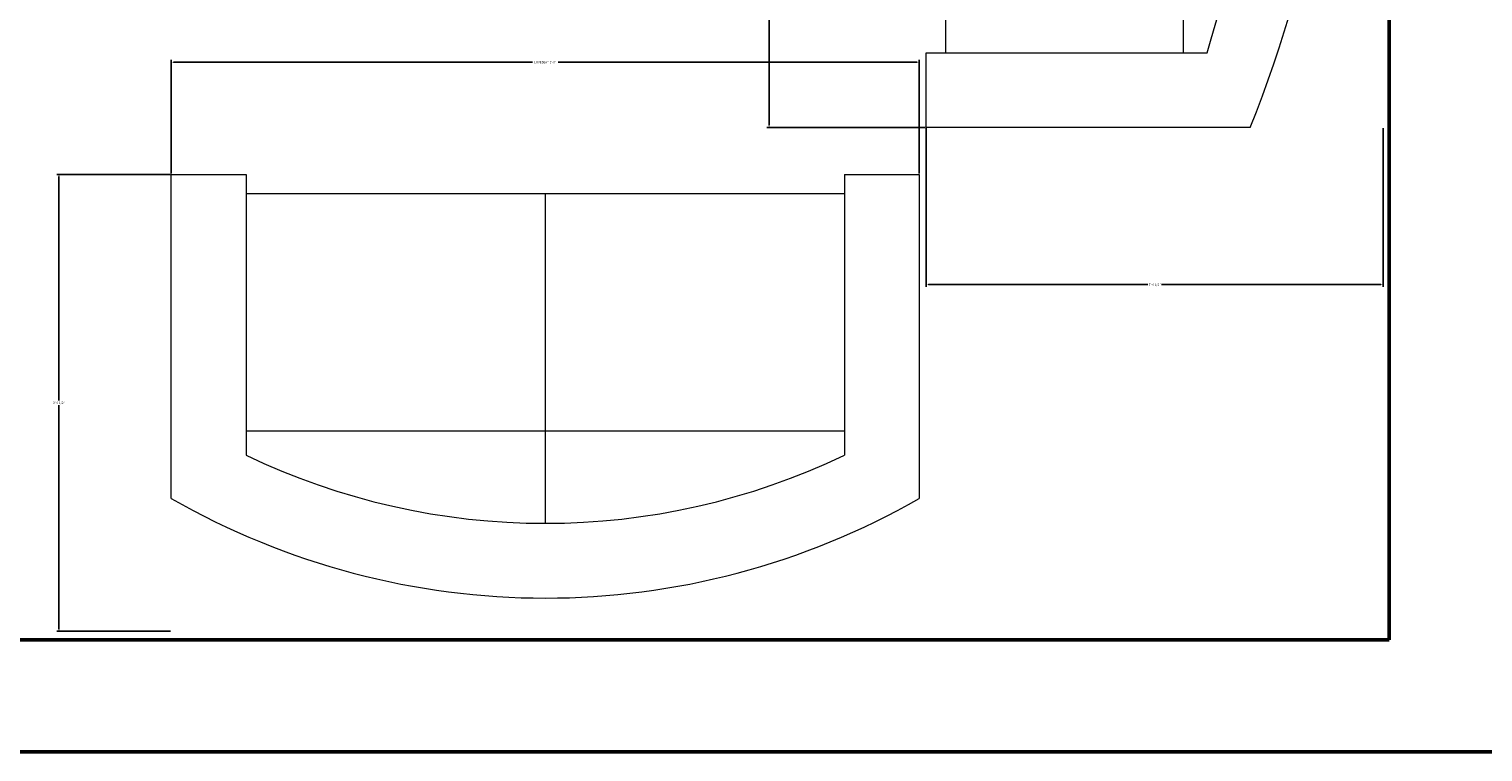
# Model space of a CAD drawing. Units: inches. Extents: x -105 to 1196, y -792 to 119.
# Tile 11 of 23: x 206 to 322, y -438 to -380. Entities that reach past the tile are written whole.
import ezdxf

# ---------------------------------------------------------------- set-up
doc = ezdxf.new("R2010")
doc.units = ezdxf.units.IN
doc.header["$MEASUREMENT"] = 0
for name, color, linetype, lineweight in [('A-ANNO-DIMS', 2, 'Continuous', 18), ('A-FURN', 8, 'Continuous', 18), ('A-WALL', 3, 'Continuous', 50)]:
    doc.layers.add(name, color=color, linetype=linetype, lineweight=lineweight)
doc.styles.get("Standard").update_dxf_attribs({"font": 'arial.ttf'})
doc.dimstyles.get("Standard").update_dxf_attribs({"dimtxt": 0.18, "dimasz": 0.18, "dimexe": 0.18, "dimexo": 0.0625, "dimgap": 0.09, "dimtad": 0, "dimtih": 1, "dimtoh": 1, "dimdec": 1, "dimzin": 0, "dimdsep": 46, "dimlunit": 4, "dimtxsty": 'Standard', "dimcen": 0.09, "dimadec": 0, "dimazin": 0, "dimtfac": 1, "dimtdec": 1, "dimtofl": 0, "dimtmove": 0, "dimatfit": 3, "dimfxl": 1, "dimtolj": 1, "dimtzin": 0, "dimarcsym": 0})

# ---------------------------------------------------------------- blocks, each defined once
blk = doc.blocks.new('Sofa - Roundback 7 ft.')
for p, q in [((-12.00002, -32.4421), (-12.00003, -6.5971)), ((11.99997, -32.4421), (11.99998, -6.5971)), ((-36.000027, -34), (-36.000027, -11.4696)), ((35.99998, -34), (35.99998, -11.4696)), ((-35.999844, -13.3819), (35.9998, -13.3819)), ((-36.000027, -32.4421), (35.99998, -32.4421))]:
    blk.add_line(p, q)
for points in [[(-36.000027, -34), (-42.000027, -34), (-42.000027, -8)], [(41.99998, -8), (41.99998, -34), (35.99998, -34)]]:
    blk.add_lwpolyline(points)
for centre, radius, start, end in [((0, -114.25), 114.25, 68.43141, 111.5686), ((-0.00001, -127.1968), 121.1968, 72.72033, 107.2797)]:
    blk.add_arc(centre, radius, start, end)
blk = doc.blocks.new('Sofa - Roundback Loveseat 5 ft.')
for p, q in [((0, -32.44198), (0, -5.99998)), ((-24, -33.99998), (-24, -11.46958)), ((24.00004, -33.99998), (24.00004, -11.46958)), ((-23.9998, -13.38178), (23.99986, -13.38178)), ((-24, -32.44198), (24.00004, -32.44198))]:
    blk.add_line(p, q)
for points in [[(-24, -33.99998), (-30, -33.99998), (-30, -7.99998)], [(30.00004, -7.99998), (30.00004, -33.99998), (24.00004, -33.99998)]]:
    blk.add_lwpolyline(points)
for centre, radius, start, end in [((0, -60.24998), 60.24998, 60.13715, 119.8628), ((0, -61.38438), 55.38444, 64.32083, 115.6792)]:
    blk.add_arc(centre, radius, start, end)
blk = doc.blocks.new('*D77')
at = {"layer": 'A-ANNO-DIMS', "color": 0, "lineweight": -2, "transparency": 16777216}
for p, q in [((277.54, -304.12), (264.83, -304.12)), ((265.01, -304.3), (265.01, -345.94)), ((265.01, -387.94), (265.01, -346.31)), ((277.54, -388.12), (264.83, -388.12))]:
    blk.add_line(p, q, dxfattribs=at)
at = {"layer": 'A-ANNO-DIMS', "color": 0, "transparency": 16777216}
for points in [[(264.98, -304.3), (265.04, -304.3), (265.01, -304.12)], [(264.98, -387.94), (265.04, -387.94), (265.01, -388.12)]]:
    blk.add_solid(points, dxfattribs=at)
at = {"layer": 'Defpoints', "color": 0, "transparency": 16777216}
for p in [(277.61, -304.12), (265.01, -388.12), (277.61, -388.12)]:
    blk.add_point(p, dxfattribs=at)
at = {"layer": 'A-ANNO-DIMS', "color": 0, "transparency": 16777216, "insert": (265.01, -346.12), "char_height": 0.18, "attachment_point": 5}
blk.add_mtext('\\A1;SOFA 7\'-0"', dxfattribs=at)
blk = doc.blocks.new('*D78')
at = {"layer": 'A-ANNO-DIMS', "color": 0, "lineweight": -2, "transparency": 16777216}
for p, q in [((277.61, -388.18), (277.61, -400.9)), ((314.27, -388.18), (314.27, -400.9)), ((277.79, -400.72), (295.4, -400.72)), ((314.09, -400.72), (296.48, -400.72))]:
    blk.add_line(p, q, dxfattribs=at)
at = {"layer": 'A-ANNO-DIMS', "color": 0, "transparency": 16777216}
for points in [[(277.79, -400.69), (277.79, -400.75), (277.61, -400.72)], [(314.09, -400.69), (314.09, -400.75), (314.27, -400.72)]]:
    blk.add_solid(points, dxfattribs=at)
at = {"layer": 'Defpoints', "color": 0, "transparency": 16777216}
for p in [(277.61, -388.12), (314.27, -388.12), (314.27, -400.72)]:
    blk.add_point(p, dxfattribs=at)
at = {"layer": 'A-ANNO-DIMS', "color": 0, "transparency": 16777216, "insert": (295.94, -400.72), "char_height": 0.18, "attachment_point": 5}
blk.add_mtext('\\A1;3\'-0 1/2"', dxfattribs=at)
blk = doc.blocks.new('*D79')
at = {"layer": 'A-ANNO-DIMS', "color": 0, "lineweight": -2, "transparency": 16777216}
for p, q in [((217.06, -391.82), (217.06, -382.7)), ((217.24, -382.88), (246.04, -382.88)), ((276.88, -382.88), (248.09, -382.88)), ((277.06, -391.82), (277.06, -382.7))]:
    blk.add_line(p, q, dxfattribs=at)
at = {"layer": 'A-ANNO-DIMS', "color": 0, "transparency": 16777216}
for points in [[(217.24, -382.85), (217.24, -382.91), (217.06, -382.88)], [(276.88, -382.85), (276.88, -382.91), (277.06, -382.88)]]:
    blk.add_solid(points, dxfattribs=at)
at = {"layer": 'Defpoints', "color": 0, "transparency": 16777216}
for p in [(217.06, -382.88), (217.06, -391.88), (277.06, -391.88)]:
    blk.add_point(p, dxfattribs=at)
at = {"layer": 'A-ANNO-DIMS', "color": 0, "transparency": 16777216, "insert": (247.06, -382.88), "char_height": 0.18, "attachment_point": 5}
blk.add_mtext('\\A1;LOVESEAT 5\'-0"', dxfattribs=at)
blk = doc.blocks.new('*D80')
at = {"layer": 'A-ANNO-DIMS', "color": 0, "lineweight": -2, "transparency": 16777216}
for p, q in [((217, -391.88), (207.88, -391.88)), ((208.06, -392.06), (208.06, -410.03)), ((208.06, -428.37), (208.06, -410.39)), ((217, -428.55), (207.88, -428.55))]:
    blk.add_line(p, q, dxfattribs=at)
at = {"layer": 'A-ANNO-DIMS', "color": 0, "transparency": 16777216}
for points in [[(208.03, -392.06), (208.09, -392.06), (208.06, -391.88)], [(208.03, -428.37), (208.09, -428.37), (208.06, -428.55)]]:
    blk.add_solid(points, dxfattribs=at)
at = {"layer": 'Defpoints', "color": 0, "transparency": 16777216}
for p in [(217.06, -391.88), (208.06, -428.55), (217.06, -428.55)]:
    blk.add_point(p, dxfattribs=at)
at = {"layer": 'A-ANNO-DIMS', "color": 0, "transparency": 16777216, "insert": (208.06, -410.21), "char_height": 0.18, "attachment_point": 5}
blk.add_mtext('\\A1;3\'-0 1/2"', dxfattribs=at)

msp = doc.modelspace()

# ---------------------------------------------------------------- linework, layer by layer
at = {"layer": 'A-WALL'}
for p, q in [((314.74, -268.11), (314.74, -429.23)), ((188.8, -429.23), (314.74, -429.23)), ((188.8, -438.23), (323.74, -438.23))]:
    msp.add_line(p, q, dxfattribs=at)

# ---------------------------------------------------------------- block references
at = {"layer": 'A-FURN'}
for name, p, rotation in [('Sofa - Roundback 7 ft.', (311.61, -346.12), 270), ('Sofa - Roundback Loveseat 5 ft.', (247.06, -425.88), 180)]:
    msp.add_blockref(name, p, dxfattribs=dict(at, rotation=rotation))

# ---------------------------------------------------------------- dimensions: what is measured, and where the dimension line sits
at = {"layer": 'A-ANNO-DIMS'}
for base, p1, p2, angle, text, picture, middle in [((265.01, -388.12), (277.61, -304.12), (277.61, -388.12), 270, 'SOFA <>', '*D77', (265.01, -346.12)), ((217.06, -382.88), (277.06, -391.88), (217.06, -391.88), 180, 'LOVESEAT <>', '*D79', (247.06, -382.88))]:
    dim = msp.add_linear_dim(base=base, p1=p1, p2=p2, angle=angle, text=text, dimstyle='Standard', override={"dimdec": 1, "dimlfac": 1, "dimrnd": 0, "dimzin": 1, "dimdsep": 46, "dimlunit": 4, "dimfrac": 2}, dxfattribs=at)
    dim.commit()
    dim.dimension.update_dxf_attribs({"geometry": picture, "text_midpoint": middle})
dim = msp.add_linear_dim(base=(314.27, -400.72), p1=(277.61, -388.12), p2=(314.27, -388.12), dimstyle='Standard', override={"dimdec": 1, "dimlfac": 1, "dimrnd": 0, "dimzin": 1, "dimdsep": 46, "dimlunit": 4, "dimfrac": 2}, dxfattribs=at)
dim.commit()
dim.dimension.update_dxf_attribs({"geometry": '*D78', "text_midpoint": (295.94, -400.72)})
dim = msp.add_linear_dim(base=(208.06, -428.55), p1=(217.06, -391.88), p2=(217.06, -428.55), angle=270, dimstyle='Standard', override={"dimdec": 1, "dimlfac": 1, "dimrnd": 0, "dimzin": 1, "dimdsep": 46, "dimlunit": 4, "dimfrac": 2}, dxfattribs=at)
dim.commit()
dim.dimension.update_dxf_attribs({"geometry": '*D80', "text_midpoint": (208.06, -410.21)})

doc.saveas('drawing.dxf')
